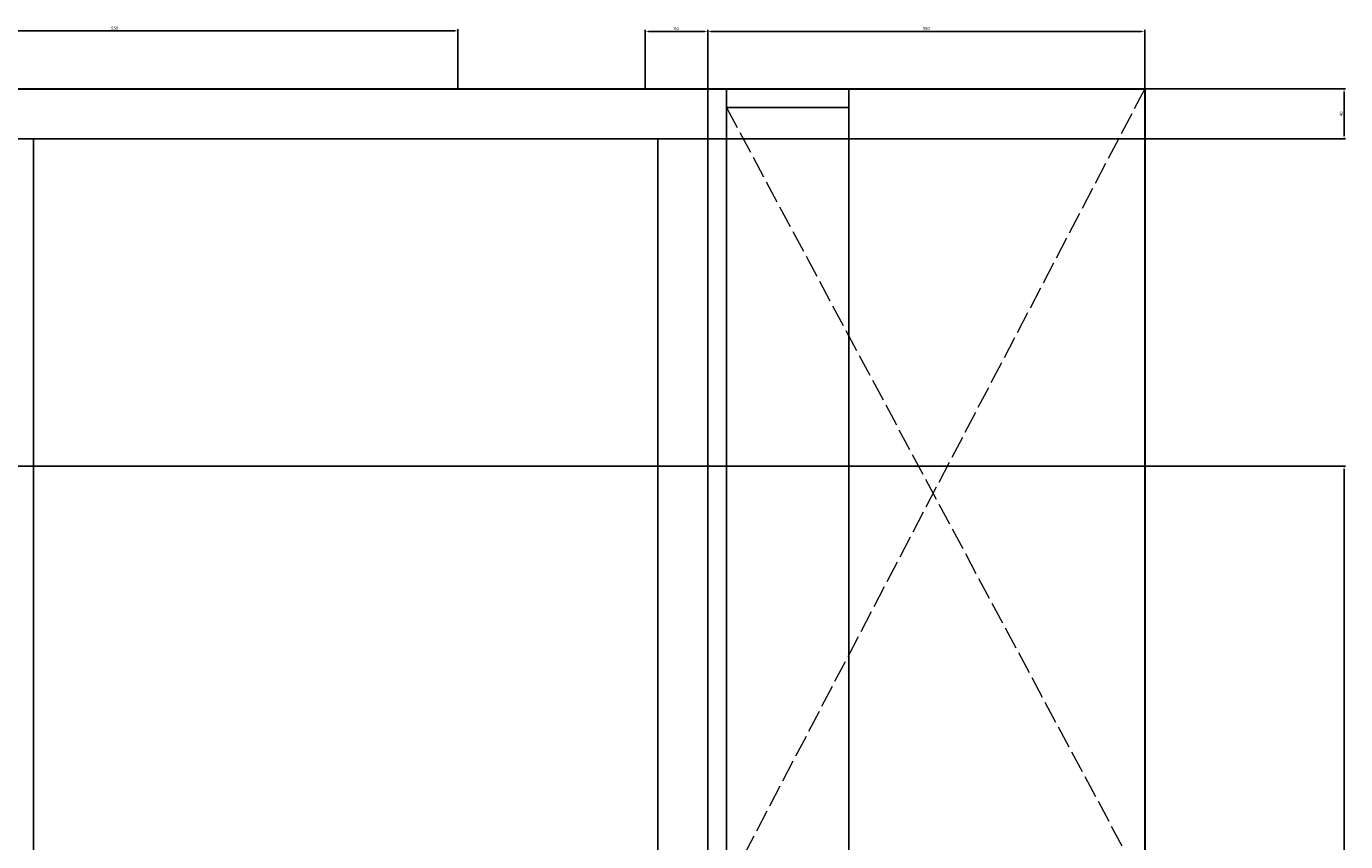
# Model space of a CAD drawing. Units: millimetres. Extents: x 2332 to 5836, y -853 to 2199.
# Tile 16 of 16: x 4779 to 5836, y 1405 to 2058. Entities that reach past the tile are written whole.
import ezdxf

# ---------------------------------------------------------------- set-up
doc = ezdxf.new("R2010")
doc.units = ezdxf.units.MM
doc.linetypes.add('ACAD_ISO02W100', pattern=[15, 12, -3])
doc.layers.get('0').update_dxf_attribs({"color": 8})
for name, color, linetype, lineweight in [('A-ANNO-DIMS', 2, 'Continuous', 18), ('A-CSWK-HIDN', 8, 'ACAD_ISO02W100', 13), ('A-WALL', 8, 'Continuous', 30), ('SHELF', 40, 'Continuous', 25)]:
    doc.layers.add(name, color=color, linetype=linetype, lineweight=lineweight)
doc.styles.get("Standard").update_dxf_attribs({"font": 'arial.ttf'})
doc.dimstyles.new('ISO-25', dxfattribs={"dimtxt": 2.5, "dimasz": 2.5, "dimexe": 1.25, "dimexo": 0.625, "dimtad": 1, "dimtxsty": 'Standard', "dimcen": 2.5, "dimadec": 0, "dimazin": 0, "dimtfac": 1, "dimtmove": 0, "dimatfit": 3, "dimfxl": 1, "dimarcsym": 0})

# ---------------------------------------------------------------- blocks, each defined once
blk = doc.blocks.new('*D5')
at = {"layer": 'A-ANNO-DIMS', "color": 0, "lineweight": -2, "transparency": 16777216}
for p, q in [((4575, 2008.4), (4575, 2055.5)), ((4577.5, 2054.2), (5122.5, 2054.2)), ((5125, 2008.4), (5125, 2055.5))]:
    blk.add_line(p, q, dxfattribs=at)
at = {"layer": 'A-ANNO-DIMS', "color": 0, "transparency": 16777216}
for points in [[(4577.5, 2054.7), (4577.5, 2053.8), (4575, 2054.2)], [(5122.5, 2054.7), (5122.5, 2053.8), (5125, 2054.2)]]:
    blk.add_solid(points, dxfattribs=at)
at = {"layer": 'Defpoints', "color": 0, "transparency": 16777216}
for p in [(5125, 2054.2), (4575, 2007.8), (5125, 2007.8)]:
    blk.add_point(p, dxfattribs=at)
at = {"layer": 'A-ANNO-DIMS', "color": 0, "transparency": 16777216, "insert": (4850, 2056.1), "char_height": 2.5, "attachment_point": 5}
blk.add_mtext('550', dxfattribs=at)
blk = doc.blocks.new('*D6')
at = {"layer": 'A-ANNO-DIMS', "color": 0, "lineweight": -2, "transparency": 16777216}
for p, q in [((5325, 2008.4), (5325, 2055.1)), ((5672.5, 2053.8), (5327.5, 2053.8)), ((5675, 2008.4), (5675, 2055.1))]:
    blk.add_line(p, q, dxfattribs=at)
at = {"layer": 'A-ANNO-DIMS', "color": 0, "transparency": 16777216}
for points in [[(5327.5, 2054.2), (5327.5, 2053.4), (5325, 2053.8)], [(5672.5, 2054.2), (5672.5, 2053.4), (5675, 2053.8)]]:
    blk.add_solid(points, dxfattribs=at)
at = {"layer": 'Defpoints', "color": 0, "transparency": 16777216}
for p in [(5325, 2053.8), (5325, 2007.8), (5675, 2007.8)]:
    blk.add_point(p, dxfattribs=at)
at = {"layer": 'A-ANNO-DIMS', "color": 0, "transparency": 16777216, "insert": (5500, 2055.7), "char_height": 2.5, "attachment_point": 5}
blk.add_mtext('350', dxfattribs=at)
blk = doc.blocks.new('*D7')
at = {"layer": 'A-ANNO-DIMS', "color": 0, "lineweight": -2, "transparency": 16777216}
for p, q in [((5275, 2008.4), (5275, 2055.1)), ((5322.5, 2053.8), (5277.5, 2053.8)), ((5325, 2008.4), (5325, 2055.1))]:
    blk.add_line(p, q, dxfattribs=at)
at = {"layer": 'A-ANNO-DIMS', "color": 0, "transparency": 16777216}
for points in [[(5277.5, 2054.2), (5277.5, 2053.4), (5275, 2053.8)], [(5322.5, 2054.2), (5322.5, 2053.4), (5325, 2053.8)]]:
    blk.add_solid(points, dxfattribs=at)
at = {"layer": 'Defpoints', "color": 0, "transparency": 16777216}
for p in [(5275, 2053.8), (5275, 2007.8), (5325, 2007.8)]:
    blk.add_point(p, dxfattribs=at)
at = {"layer": 'A-ANNO-DIMS', "color": 0, "transparency": 16777216, "insert": (5300, 2055.7), "char_height": 2.5, "attachment_point": 5}
blk.add_mtext('50', dxfattribs=at)
blk = doc.blocks.new('CAB-END-STILE')
for p, q in [((0, 1240), (0, 600)), ((98.1, 1240), (98.1, 0)), ((113.1, 1240), (113.1, 0)), ((98.1, 1225), (0, 1225)), ((0, 615), (98.1, 615))]:
    blk.add_line(p, q)
blk = doc.blocks.new('*D21')
at = {"layer": 'A-ANNO-DIMS', "color": 0, "lineweight": -2, "transparency": 16777216}
for p, q in [((5325.7, 2007.8), (5835.9, 2007.8)), ((5834.7, 2005.3), (5834.7, 1970.3)), ((5325.7, 1967.8), (5835.9, 1967.8))]:
    blk.add_line(p, q, dxfattribs=at)
at = {"layer": 'A-ANNO-DIMS', "color": 0, "transparency": 16777216}
for points in [[(5834.3, 2005.3), (5835.1, 2005.3), (5834.7, 2007.8)], [(5834.3, 1970.3), (5835.1, 1970.3), (5834.7, 1967.8)]]:
    blk.add_solid(points, dxfattribs=at)
at = {"layer": 'Defpoints', "color": 0, "transparency": 16777216}
for p in [(5325, 2007.8), (5325, 1967.8), (5834.7, 1967.8)]:
    blk.add_point(p, dxfattribs=at)
at = {"layer": 'A-ANNO-DIMS', "color": 0, "transparency": 16777216, "insert": (5832.8, 1987.8), "char_height": 2.5, "attachment_point": 5, "rotation": 90}
blk.add_mtext('40', dxfattribs=at)
blk = doc.blocks.new('*D25')
at = {"layer": 'A-ANNO-DIMS', "color": 0, "lineweight": -2, "transparency": 16777216}
for p, q in [((4341.5, 1705.8), (5835.9, 1705.8)), ((5834.7, 1032.3), (5834.7, 1703.3)), ((4341.5, 1029.8), (5835.9, 1029.8))]:
    blk.add_line(p, q, dxfattribs=at)
at = {"layer": 'A-ANNO-DIMS', "color": 0, "transparency": 16777216}
for points in [[(5834.3, 1703.3), (5835.1, 1703.3), (5834.7, 1705.8)], [(5834.3, 1032.3), (5835.1, 1032.3), (5834.7, 1029.8)]]:
    blk.add_solid(points, dxfattribs=at)
at = {"layer": 'Defpoints', "color": 0, "transparency": 16777216}
for p in [(4340.9, 1705.8), (5834.7, 1705.8), (4340.9, 1029.8)]:
    blk.add_point(p, dxfattribs=at)
at = {"layer": 'A-ANNO-DIMS', "color": 0, "transparency": 16777216, "insert": (5832.8, 1367.8), "char_height": 2.5, "attachment_point": 5, "rotation": 90}
blk.add_mtext('676', dxfattribs=at)

msp = doc.modelspace()

# ---------------------------------------------------------------- linework, layer by layer
at = {"layer": 'A-CSWK-HIDN', "ltscale": 1.5}
for p, q in [((5675.04, 2007.803), (5340.04, 1367.803)), ((5340.04, 1992.803), (5675.04, 1367.803))]:
    msp.add_line(p, q, dxfattribs=at)
at = {"layer": 'A-WALL'}
for p, q in [((4575.04, 2007.803), (5125.04, 2007.803)), ((5125.04, 2007.803), (5175.04, 2007.803)), ((5175.04, 2007.803), (5525.04, 2007.803)), ((5525.04, 2007.803), (5675.04, 2007.803)), ((5675.04, 2007.803), (5675.04, 1967.803)), ((5675.04, 1967.803), (5675.04, 1367.803))]:
    msp.add_line(p, q, dxfattribs=at)
at = {"layer": 'SHELF'}
for p, q in [((3095.04, 1967.803), (4785.04, 1967.803)), ((5325.04, 1967.803), (4785.04, 1967.803)), ((4785.04, 767.803), (4785.04, 1967.803)), ((5285.04, 1967.803), (5285.04, 767.803))]:
    msp.add_line(p, q, dxfattribs=at)

# ---------------------------------------------------------------- block references
at = {"layer": 'SHELF', "extrusion": (0, 0, -1), "zscale": -1}
msp.add_blockref('CAB-END-STILE', (-5438.13, 767.803), dxfattribs=at)

# ---------------------------------------------------------------- dimensions: what is measured, and where the dimension line sits
at = {"layer": 'A-ANNO-DIMS'}
for base, p1, p2, picture, middle in [((5125.04, 2054.248), (4575.04, 2007.803), (5125.04, 2007.803), '*D5', (4850.04, 2056.149)), ((5275.04, 2053.831), (5325.04, 2007.803), (5275.04, 2007.803), '*D7', (5300.04, 2055.733)), ((5325.04, 2053.831), (5675.04, 2007.803), (5325.04, 2007.803), '*D6', (5500.04, 2055.734))]:
    dim = msp.add_linear_dim(base=base, p1=p1, p2=p2, dimstyle='ISO-25', override={"dimclrd": 0, "dimclre": 0, "dimclrt": 0}, dxfattribs=at)
    dim.commit()
    dim.dimension.update_dxf_attribs({"geometry": picture, "text_midpoint": middle})
for base, p1, p2, picture, middle in [((5834.69, 1967.803), (5325.04, 2007.803), (5325.04, 1967.803), '*D21', (5832.788, 1987.803)), ((5834.69, 1705.805), (4340.894, 1029.801), (4340.894, 1705.805), '*D25', (5832.788, 1367.803))]:
    dim = msp.add_linear_dim(base=base, p1=p1, p2=p2, angle=90, dimstyle='ISO-25', override={"dimdec": 0, "dimlfac": 1, "dimrnd": 0, "dimzin": 0, "dimdsep": 46, "dimlunit": 2}, dxfattribs=at)
    dim.commit()
    dim.dimension.update_dxf_attribs({"geometry": picture, "text_midpoint": middle})

doc.saveas('drawing.dxf')
